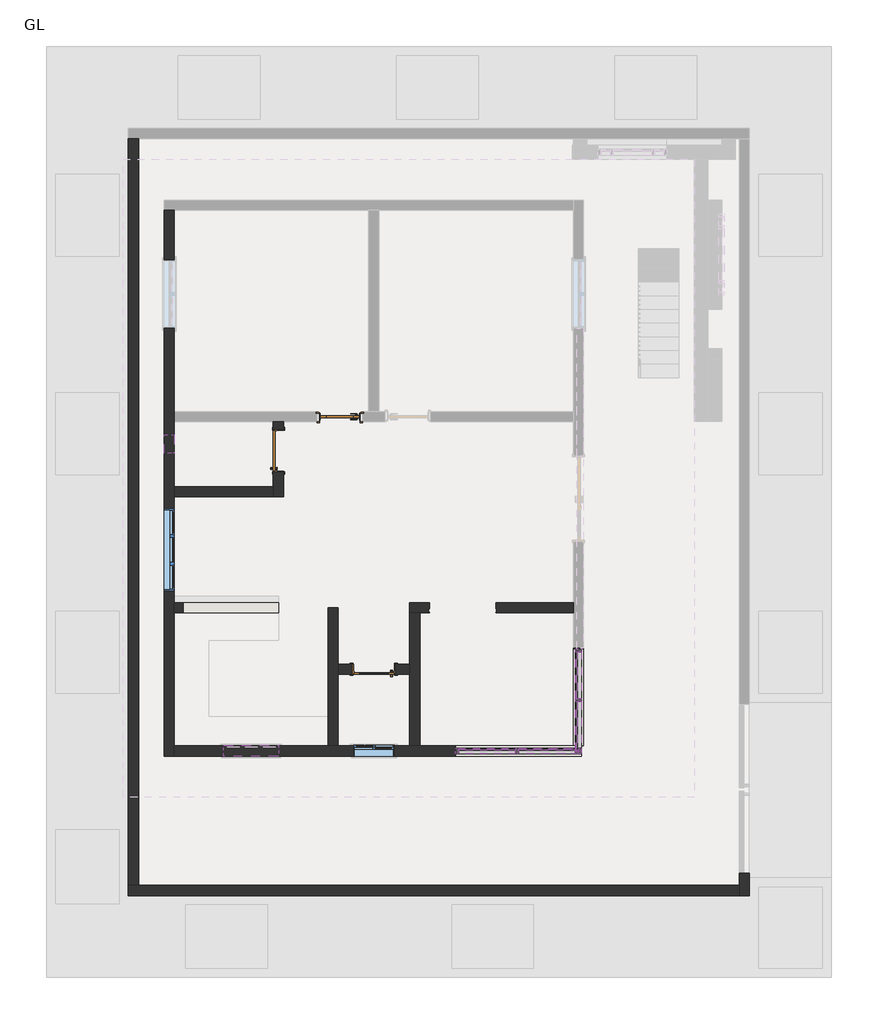
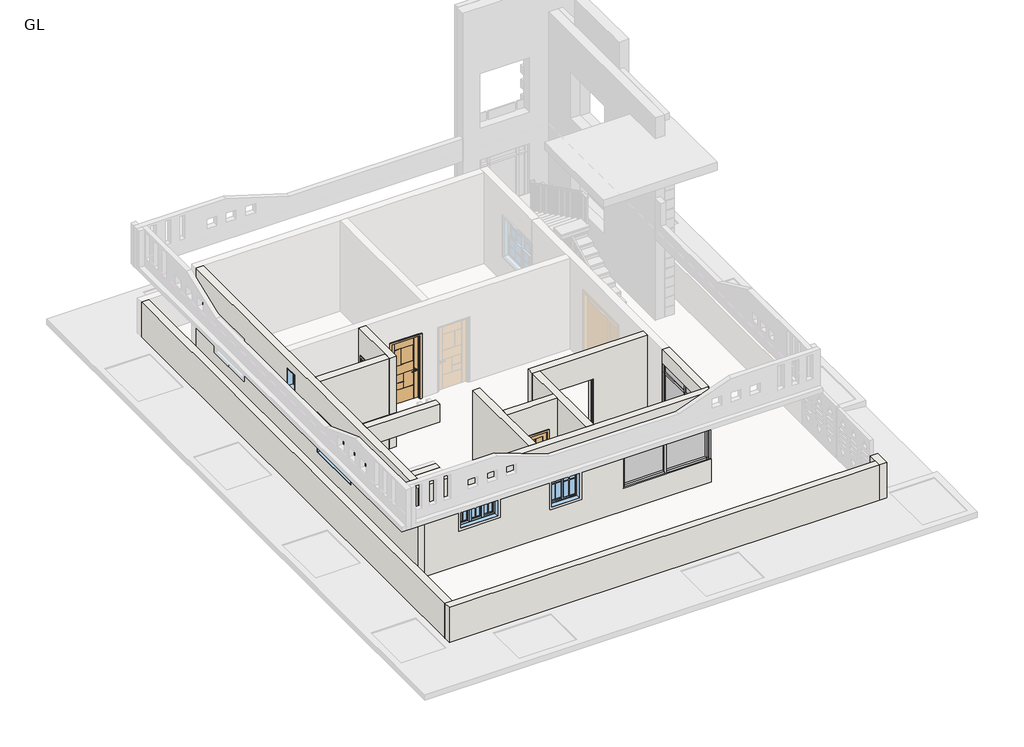
# One storey, part 1 of 4: 24 members, 13 walls, 8 plates, 4 windows, 3 doors.
"""IFC4 building model written with IfcOpenShell, lengths in millimetres."""

from ifc_helpers import new_model, si_unit, frame, origin, origin_with_axes, place, context, project, spatial, polyline, outline, extrude, faceted_brep, transform, mapped, element, save
from components import door_1d7b229f, door_d5d480c1, single_modern_wooden_door_17379_single_modern_wooden_door_9761f21e, member_cba00588, member_58fbc06e, member_82905deb, member_75d1e245, member_3c3dc66a, member_4491d118, member_78934672, member_697f972d, member_ecafcbb3, member_c327c56d, member_aaf6ec4e, member_7ce6cacc, member_69204bcc, member_41dcc1f0, system_panel_glazed_27c3d98e, system_panel_glazed_8e393102, system_panel_glazed_36abd0f2, system_panel_glazed_6ba3ac31, system_panel_glazed_448caaff, system_panel_glazed_d7074436, system_panel_glazed_2854df63, system_panel_glazed_f3e19b1d, window_aa618e30, window_06177765, window_dd70d674, window_fdfe0ef3

model = new_model("IFC4")

# Units and contexts
model_context = context("Model", 3, world=origin())
ifc_project = project(units=[si_unit("LENGTHUNIT", "METRE", prefix="MILLI")], contexts=[model_context])

# Site, building, storey
site = spatial("IfcSite", under=ifc_project)
building = spatial("IfcBuilding", under=site)
storey = spatial("IfcBuildingStorey", under=building, Name="GL", Elevation=0.0)

# Doors
placement = place(None, origin())
door_shape = door_1d7b229f(model_context)
element("IfcDoor", 1, ObjectType="Door-Interior-Single-Flush_Panel-Wood : 36\" x 84\"", at=placement, inside=storey, context=model_context, shape_type="MappedRepresentation", body=[
    mapped(door_shape, transform((-9036.4027598, 5465.7342801, 0.0), x_axis=(0.0, 1.0, 0.0), y_axis=(-1.0, 0.0, 0.0), z_axis=(0.0, 0.0, 1.0))),
])
door_2_shape = door_d5d480c1(model_context)
element("IfcDoor", 2, ObjectType="Door-Interior-Single-Full Glass-Wood : 36\" x 80\"", at=placement, inside=storey, context=model_context, shape_type="MappedRepresentation", body=[
    mapped(door_2_shape, transform((-6899.6277598, 585.7592801, 0.0), x_axis=(-1.0, 0.0, 0.0), y_axis=(0.0, -1.0, 0.0), z_axis=(0.0, 0.0, 1.0))),
])
single_modern_wooden_door_17379_single_modern_wooden_door_shape = single_modern_wooden_door_17379_single_modern_wooden_door_9761f21e(model_context)
element("IfcDoor", 3, ObjectType="Single_-_Modern_Wooden_Door_17379 : Single_-_Modern_Wooden_Door_17379", at=placement, inside=storey, context=model_context, shape_type="MappedRepresentation", body=[
    mapped(single_modern_wooden_door_17379_single_modern_wooden_door_shape, transform((-7661.6277598, 6227.7342801, 0.0), x_axis=(1.0, 0.0, 0.0), y_axis=(0.0, 1.0, 0.0), z_axis=(0.0, 0.0, 1.0))),
])

# Members
member_shape = member_cba00588(model_context)
element("IfcMember", 4, ObjectType="Rectangular Mullion : 2.5\" x 5\" rectangular", at=placement, inside=storey, context=model_context, shape_type="MappedRepresentation", body=[
    mapped(member_shape, transform((-3730.9777598, -1239.8657199, 2590.8), x_axis=(0.0, 0.0, 1.0), y_axis=(0.0, -1.0, 0.0), z_axis=(1.0, 0.0, 0.0))),
])
element("IfcMember", 5, ObjectType="Rectangular Mullion : 2.5\" x 5\" rectangular", at=placement, inside=storey, context=model_context, shape_type="MappedRepresentation", body=[
    mapped(member_shape, transform((-5007.3277598, -1239.8657199, 762.0), x_axis=(0.0, 0.0, -1.0), y_axis=(0.0, -1.0, 0.0), z_axis=(-1.0, 0.0, 0.0))),
])
member_2_shape = member_58fbc06e(model_context)
element("IfcMember", 6, ObjectType="Rectangular Mullion : 2.5\" x 5\" rectangular", at=placement, inside=storey, context=model_context, shape_type="MappedRepresentation", body=[
    mapped(member_2_shape, transform((-3730.9777598, -1239.8657199, 2286.0), x_axis=(0.0, 0.0, 1.0), y_axis=(0.0, -1.0, 0.0), z_axis=(1.0, 0.0, 0.0))),
])
member_3_shape = member_82905deb(model_context)
element("IfcMember", 7, ObjectType="Rectangular Mullion : 2.5\" x 5\" rectangular", at=placement, inside=storey, context=model_context, shape_type="MappedRepresentation", body=[
    mapped(member_3_shape, transform((-3699.2277598, -1239.8657199, 762.0), x_axis=(1.0, 0.0, 0.0), y_axis=(0.0, -1.0, 0.0), z_axis=(0.0, 0.0, -1.0))),
])
element("IfcMember", 8, ObjectType="Rectangular Mullion : 2.5\" x 5\" rectangular", at=placement, inside=storey, context=model_context, shape_type="MappedRepresentation", body=[
    mapped(member_3_shape, transform((-2327.6277598, -96.8657199, 762.0), x_axis=(0.0, 1.0, 0.0), y_axis=(1.0, 0.0, 0.0), z_axis=(0.0, 0.0, -1.0))),
])
member_4_shape = member_75d1e245(model_context)
element("IfcMember", 9, ObjectType="Rectangular Mullion : 2.5\" x 5\" rectangular", at=placement, inside=storey, context=model_context, shape_type="MappedRepresentation", body=[
    mapped(member_4_shape, transform((-3699.2277598, -1239.8657199, 2286.0), x_axis=(1.0, 0.0, 0.0), y_axis=(0.0, -1.0, 0.0), z_axis=(0.0, 0.0, -1.0))),
])
element("IfcMember", 10, ObjectType="Rectangular Mullion : 2.5\" x 5\" rectangular", at=placement, inside=storey, context=model_context, shape_type="MappedRepresentation", body=[
    mapped(member_4_shape, transform((-2327.6277598, -96.8657199, 2286.0), x_axis=(0.0, 1.0, 0.0), y_axis=(1.0, 0.0, 0.0), z_axis=(0.0, 0.0, -1.0))),
])
member_5_shape = member_3c3dc66a(model_context)
element("IfcMember", 11, ObjectType="Rectangular Mullion : 2.5\" x 5\" rectangular", at=placement, inside=storey, context=model_context, shape_type="MappedRepresentation", body=[
    mapped(member_5_shape, transform((-5070.8277598, -1239.8657199, 2590.8), x_axis=(-1.0, 0.0, 0.0), y_axis=(0.0, -1.0, 0.0), z_axis=(0.0, 0.0, 1.0))),
])
element("IfcMember", 12, ObjectType="Rectangular Mullion : 2.5\" x 5\" rectangular", at=placement, inside=storey, context=model_context, shape_type="MappedRepresentation", body=[
    mapped(member_5_shape, transform((-2327.6277598, -1303.3657199, 2590.8), x_axis=(0.0, -1.0, 0.0), y_axis=(1.0, 0.0, 0.0), z_axis=(0.0, 0.0, 1.0))),
])
member_6_shape = member_4491d118(model_context)
element("IfcMember", 13, ObjectType="Rectangular Mullion : 2.5\" x 5\" rectangular", at=placement, inside=storey, context=model_context, shape_type="MappedRepresentation", body=[
    mapped(member_6_shape, transform((-2327.6277598, 1046.1342801, 762.0), x_axis=(0.0, 1.0, 0.0), y_axis=(1.0, 0.0, 0.0), z_axis=(0.0, 0.0, -1.0))),
])
element("IfcMember", 14, ObjectType="Rectangular Mullion : 2.5\" x 5\" rectangular", at=placement, inside=storey, context=model_context, shape_type="MappedRepresentation", body=[
    mapped(member_5_shape, transform((-2327.6277598, 1046.1342801, 2286.0), x_axis=(0.0, 1.0, 0.0), y_axis=(1.0, 0.0, 0.0), z_axis=(0.0, 0.0, -1.0))),
])
element("IfcMember", 15, ObjectType="Rectangular Mullion : 2.5\" x 5\" rectangular", at=placement, inside=storey, context=model_context, shape_type="MappedRepresentation", body=[
    mapped(member_6_shape, transform((-5070.8277598, -1239.8657199, 2286.0), x_axis=(-1.0, 0.0, 0.0), y_axis=(0.0, -1.0, 0.0), z_axis=(0.0, 0.0, 1.0))),
])
element("IfcMember", 16, ObjectType="Rectangular Mullion : 2.5\" x 5\" rectangular", at=placement, inside=storey, context=model_context, shape_type="MappedRepresentation", body=[
    mapped(member_6_shape, transform((-2327.6277598, -1303.3657199, 2286.0), x_axis=(0.0, -1.0, 0.0), y_axis=(1.0, 0.0, 0.0), z_axis=(0.0, 0.0, 1.0))),
])
member_7_shape = member_78934672(model_context)
element("IfcMember", 17, ObjectType="Rectangular Mullion : 2.5\" x 5\" rectangular", at=placement, inside=storey, context=model_context, shape_type="MappedRepresentation", body=[
    mapped(member_7_shape, transform((-2327.6277598, 982.6342801, 2590.8), x_axis=(0.0, 0.0, 1.0), y_axis=(1.0, 0.0, 0.0), z_axis=(0.0, 1.0, 0.0))),
])
element("IfcMember", 18, ObjectType="Rectangular Mullion : 2.5\" x 5\" rectangular", at=placement, inside=storey, context=model_context, shape_type="MappedRepresentation", body=[
    mapped(member_7_shape, transform((-2327.6277598, -65.1157199, 762.0), x_axis=(0.0, 0.0, -1.0), y_axis=(1.0, 0.0, 0.0), z_axis=(0.0, -1.0, 0.0))),
])
member_8_shape = member_697f972d(model_context)
element("IfcMember", 19, ObjectType="Rectangular Mullion : 2.5\" x 5\" rectangular", at=placement, inside=storey, context=model_context, shape_type="MappedRepresentation", body=[
    mapped(member_8_shape, transform((-2327.6277598, 982.6342801, 2286.0), x_axis=(0.0, 0.0, 1.0), y_axis=(1.0, 0.0, 0.0), z_axis=(0.0, 1.0, 0.0))),
])
member_9_shape = member_ecafcbb3(model_context)
element("IfcMember", 20, ObjectType="Rectangular Mullion : 2.5\" x 5\" rectangular", at=placement, inside=storey, context=model_context, shape_type="MappedRepresentation", body=[
    mapped(member_9_shape, transform((-2264.1277598, -1239.8657199, 762.0), x_axis=(1.0, 0.0, 0.0), y_axis=(0.0, -1.0, 0.0), z_axis=(0.0, 0.0, -1.0))),
])
member_10_shape = member_c327c56d(model_context)
element("IfcMember", 21, ObjectType="Rectangular Mullion : 2.5\" x 5\" rectangular", at=placement, inside=storey, context=model_context, shape_type="MappedRepresentation", body=[
    mapped(member_10_shape, transform((-2264.1277598, -1239.8657199, 2317.75), x_axis=(1.0, 0.0, 0.0), y_axis=(0.0, -1.0, 0.0), z_axis=(0.0, 0.0, -1.0))),
])
member_11_shape = member_aaf6ec4e(model_context)
element("IfcMember", 22, ObjectType="Rectangular Mullion : 2.5\" x 5\" rectangular", at=placement, inside=storey, context=model_context, shape_type="MappedRepresentation", body=[
    mapped(member_11_shape, transform((-2327.6277598, -1239.8657199, 762.0), x_axis=(0.0, 0.0, -1.0), y_axis=(1.0, 0.0, 0.0), z_axis=(0.0, -1.0, 0.0))),
])
member_12_shape = member_7ce6cacc(model_context)
element("IfcMember", 23, ObjectType="Rectangular Mullion : 2.5\" x 5\" rectangular", at=placement, inside=storey, context=model_context, shape_type="MappedRepresentation", body=[
    mapped(member_12_shape, transform((-2327.6277598, -128.6157199, 2286.0), x_axis=(0.0, 0.0, 1.0), y_axis=(1.0, 0.0, 0.0), z_axis=(0.0, 1.0, 0.0))),
])
element("IfcMember", 24, ObjectType="Rectangular Mullion : 2.5\" x 5\" rectangular", at=placement, inside=storey, context=model_context, shape_type="MappedRepresentation", body=[
    mapped(member_11_shape, transform((-2327.6277598, -128.6157199, 2590.8), x_axis=(0.0, 0.0, 1.0), y_axis=(1.0, 0.0, 0.0), z_axis=(0.0, 1.0, 0.0))),
])
member_13_shape = member_69204bcc(model_context)
element("IfcMember", 25, ObjectType="Rectangular Mullion : 2.5\" x 5\" rectangular", at=placement, inside=storey, context=model_context, shape_type="MappedRepresentation", body=[
    mapped(member_13_shape, transform((-2327.6277598, -1239.8657199, 2590.8), x_axis=(0.0, 0.0, 1.0), y_axis=(0.0, -1.0, 0.0), z_axis=(1.0, 0.0, 0.0))),
])
member_14_shape = member_41dcc1f0(model_context)
element("IfcMember", 26, ObjectType="Rectangular Mullion : 2.5\" x 5\" rectangular", at=placement, inside=storey, context=model_context, shape_type="MappedRepresentation", body=[
    mapped(member_14_shape, transform((-2264.1277598, -1239.8657199, 2286.0), x_axis=(0.0, 0.0, 1.0), y_axis=(0.0, -1.0, 0.0), z_axis=(1.0, 0.0, 0.0))),
])
element("IfcMember", 27, ObjectType="Rectangular Mullion : 2.5\" x 5\" rectangular", at=placement, inside=storey, context=model_context, shape_type="MappedRepresentation", body=[
    mapped(member_13_shape, transform((-3667.4777598, -1239.8657199, 762.0), x_axis=(0.0, 0.0, -1.0), y_axis=(0.0, -1.0, 0.0), z_axis=(-1.0, 0.0, 0.0))),
])

# Plates
system_panel_glazed_shape = system_panel_glazed_27c3d98e(model_context)
element("IfcPlate", 28, ObjectType="System Panel : Glazed", at=placement, inside=storey, context=model_context, shape_type="MappedRepresentation", body=[
    mapped(system_panel_glazed_shape, transform((-4369.1527598, -1239.8657199, 825.5), x_axis=(1.0, 0.0, 0.0), y_axis=(0.0, 1.0, 0.0), z_axis=(0.0, 0.0, 1.0))),
])
system_panel_glazed_2_shape = system_panel_glazed_8e393102(model_context)
element("IfcPlate", 29, ObjectType="System Panel : Glazed", at=placement, inside=storey, context=model_context, shape_type="MappedRepresentation", body=[
    mapped(system_panel_glazed_2_shape, transform((-4369.1527598, -1239.8657199, 2317.75), x_axis=(1.0, 0.0, 0.0), y_axis=(0.0, 1.0, 0.0), z_axis=(0.0, 0.0, 1.0))),
])
system_panel_glazed_3_shape = system_panel_glazed_36abd0f2(model_context)
element("IfcPlate", 30, ObjectType="System Panel : Glazed", at=placement, inside=storey, context=model_context, shape_type="MappedRepresentation", body=[
    mapped(system_panel_glazed_3_shape, transform((-2327.6277598, 458.7592801, 825.5), x_axis=(0.0, 1.0, 0.0), y_axis=(-1.0, 0.0, 0.0), z_axis=(0.0, 0.0, 1.0))),
])
system_panel_glazed_4_shape = system_panel_glazed_6ba3ac31(model_context)
element("IfcPlate", 31, ObjectType="System Panel : Glazed", at=placement, inside=storey, context=model_context, shape_type="MappedRepresentation", body=[
    mapped(system_panel_glazed_4_shape, transform((-2327.6277598, 458.7592801, 2317.75), x_axis=(0.0, 1.0, 0.0), y_axis=(-1.0, 0.0, 0.0), z_axis=(0.0, 0.0, 1.0))),
])
system_panel_glazed_5_shape = system_panel_glazed_448caaff(model_context)
element("IfcPlate", 32, ObjectType="System Panel : Glazed", at=placement, inside=storey, context=model_context, shape_type="MappedRepresentation", body=[
    mapped(system_panel_glazed_5_shape, transform((-2327.6277598, -684.2407199, 825.5), x_axis=(0.0, 1.0, 0.0), y_axis=(-1.0, 0.0, 0.0), z_axis=(0.0, 0.0, 1.0))),
])
system_panel_glazed_6_shape = system_panel_glazed_d7074436(model_context)
element("IfcPlate", 33, ObjectType="System Panel : Glazed", at=placement, inside=storey, context=model_context, shape_type="MappedRepresentation", body=[
    mapped(system_panel_glazed_6_shape, transform((-2327.6277598, -684.2407199, 2317.75), x_axis=(0.0, 1.0, 0.0), y_axis=(-1.0, 0.0, 0.0), z_axis=(0.0, 0.0, 1.0))),
])
system_panel_glazed_7_shape = system_panel_glazed_2854df63(model_context)
element("IfcPlate", 34, ObjectType="System Panel : Glazed", at=placement, inside=storey, context=model_context, shape_type="MappedRepresentation", body=[
    mapped(system_panel_glazed_7_shape, transform((-2997.5527598, -1239.8657199, 825.5), x_axis=(1.0, 0.0, 0.0), y_axis=(0.0, 1.0, 0.0), z_axis=(0.0, 0.0, 1.0))),
])
system_panel_glazed_8_shape = system_panel_glazed_f3e19b1d(model_context)
element("IfcPlate", 35, ObjectType="System Panel : Glazed", at=placement, inside=storey, context=model_context, shape_type="MappedRepresentation", body=[
    mapped(system_panel_glazed_8_shape, transform((-2997.5527598, -1239.8657199, 2317.75), x_axis=(1.0, 0.0, 0.0), y_axis=(0.0, 1.0, 0.0), z_axis=(0.0, 0.0, 1.0))),
])

# Walls
element("IfcWall", 36, ObjectType="Generic - 9\"", at=placement, inside=storey, context=model_context, shape_type="Brep", body=[
    faceted_brep([(-11357.3277598, -1354.1657199, 0.0), (-11357.3277598, -1125.5657199, 0.0), (-11357.3277598, 1846.2342801, 0.0), (-11357.3277598, 2074.8342801, 0.0), (-11357.3277598, 4437.0342801, 0.0), (-11357.3277598, 4665.6342801, 0.0), (-11357.3277598, 6113.4342801, 0.0), (-11357.3277598, 6342.0342801, 0.0), (-11357.3277598, 10837.8342801, 0.0), (-11357.3277598, 10837.8342801, 3048.0), (-11357.3277598, 6342.0342801, 3048.0), (-11357.3277598, 6113.4342801, 3048.0), (-11357.3277598, 4665.6342801, 3048.0), (-11357.3277598, 4437.0342801, 3048.0), (-11357.3277598, 2074.8342801, 3048.0), (-11357.3277598, 1846.2342801, 3048.0), (-11357.3277598, -1125.5657199, 3048.0), (-11357.3277598, -1354.1657199, 3048.0), (-11357.3277598, 9732.9342801, 2235.2), (-11357.3277598, 9732.9342801, 914.4), (-11357.3277598, 8208.9342801, 914.4), (-11357.3277598, 8208.9342801, 2235.2), (-11357.3277598, 2341.5342801, 2260.6), (-11357.3277598, 4170.3342801, 2260.6), (-11357.3277598, 4170.3342801, 914.4), (-11357.3277598, 2341.5342801, 914.4), (-11357.3277598, 5414.9342801, 2743.2), (-11357.3277598, 5821.3342801, 2743.2), (-11357.3277598, 5821.3342801, 2133.6), (-11357.3277598, 5414.9342801, 2133.6), (-11585.9277598, -1354.1657199, 0.0), (-11585.9277598, -1354.1657199, 3048.0), (-11585.9277598, 10837.8342801, 3048.0), (-11585.9277598, 10837.8342801, 0.0), (-11585.9277598, 9732.9342801, 2235.2), (-11585.9277598, 8208.9342801, 2235.2), (-11585.9277598, 8208.9342801, 914.4), (-11585.9277598, 9732.9342801, 914.4), (-11585.9277598, 2341.5342801, 2260.6), (-11585.9277598, 2341.5342801, 914.4), (-11585.9277598, 4170.3342801, 914.4), (-11585.9277598, 4170.3342801, 2260.6), (-11585.9277598, 5414.9342801, 2743.2), (-11585.9277598, 5414.9342801, 2133.6), (-11585.9277598, 5821.3342801, 2133.6), (-11585.9277598, 5821.3342801, 2743.2)], [[[0, 1, 2, 3, 4, 5, 6, 7, 8, 9, 10, 11, 12, 13, 14, 15, 16, 17], [18, 19, 20, 21], [22, 23, 24, 25], [26, 27, 28, 29]], [[30, 31, 32, 33], [34, 35, 36, 37], [38, 39, 40, 41], [42, 43, 44, 45]], [[8, 7, 6, 5, 4, 3, 2, 1, 0, 30, 33]], [[17, 16, 15, 14, 13, 12, 11, 10, 9, 32, 31]], [[0, 17, 31, 30]], [[9, 8, 33, 32]], [[19, 18, 34, 37]], [[20, 19, 37, 36]], [[21, 20, 36, 35]], [[18, 21, 35, 34]], [[39, 38, 22, 25]], [[40, 39, 25, 24]], [[41, 40, 24, 23]], [[38, 41, 23, 22]], [[43, 42, 26, 29]], [[44, 43, 29, 28]], [[45, 44, 28, 27]], [[42, 45, 27, 26]]]),
])
element("IfcWall", 37, ObjectType="Generic - 9\"", at=placement, inside=storey, context=model_context, shape_type="Brep", body=[
    faceted_brep([(-2264.1277598, -1125.5657199, 2590.8), (-2441.9277598, -1125.5657199, 2590.8), (-5070.8277598, -1125.5657199, 2590.8), (-5070.8277598, -1125.5657199, 762.0), (-2441.9277598, -1125.5657199, 762.0), (-2264.1277598, -1125.5657199, 762.0), (-2264.1277598, -1125.5657199, 0.0), (-2441.9277598, -1125.5657199, 0.0), (-5870.9277598, -1125.5657199, 0.0), (-6099.5277598, -1125.5657199, 0.0), (-7699.7277598, -1125.5657199, 0.0), (-7928.3277598, -1125.5657199, 0.0), (-11357.3277598, -1125.5657199, 0.0), (-11357.3277598, -1125.5657199, 3048.0), (-7928.3277598, -1125.5657199, 3048.0), (-7699.7277598, -1125.5657199, 3048.0), (-6099.5277598, -1125.5657199, 3048.0), (-5870.9277598, -1125.5657199, 3048.0), (-2441.9277598, -1125.5657199, 3048.0), (-2264.1277598, -1125.5657199, 3048.0), (-9033.2277598, -1125.5657199, 2133.6), (-10252.4277598, -1125.5657199, 2133.6), (-10252.4277598, -1125.5657199, 1219.2), (-9033.2277598, -1125.5657199, 1219.2), (-6442.4277598, -1125.5657199, 2133.6), (-7356.8277598, -1125.5657199, 2133.6), (-7356.8277598, -1125.5657199, 914.4), (-6442.4277598, -1125.5657199, 914.4), (-2264.1277598, -1354.1657199, 2590.8), (-2264.1277598, -1354.1657199, 3048.0), (-11357.3277598, -1354.1657199, 3048.0), (-11357.3277598, -1354.1657199, 0.0), (-2264.1277598, -1354.1657199, 0.0), (-2264.1277598, -1354.1657199, 762.0), (-5070.8277598, -1354.1657199, 762.0), (-5070.8277598, -1354.1657199, 2590.8), (-9033.2277598, -1354.1657199, 2133.6), (-9033.2277598, -1354.1657199, 1219.2), (-10252.4277598, -1354.1657199, 1219.2), (-10252.4277598, -1354.1657199, 2133.6), (-6442.4277598, -1354.1657199, 2133.6), (-6442.4277598, -1354.1657199, 914.4), (-7356.8277598, -1354.1657199, 914.4), (-7356.8277598, -1354.1657199, 2133.6)], [[[0, 1, 2, 3, 4, 5, 6, 7, 8, 9, 10, 11, 12, 13, 14, 15, 16, 17, 18, 19], [20, 21, 22, 23], [24, 25, 26, 27]], [[28, 29, 30, 31, 32, 33, 34, 35], [36, 37, 38, 39], [40, 41, 42, 43]], [[13, 12, 31, 30]], [[37, 36, 20, 23]], [[38, 37, 23, 22]], [[39, 38, 22, 21]], [[36, 39, 21, 20]], [[41, 40, 24, 27]], [[42, 41, 27, 26]], [[43, 42, 26, 25]], [[40, 43, 25, 24]], [[12, 11, 10, 9, 8, 7, 6, 32, 31]], [[19, 18, 17, 16, 15, 14, 13, 30, 29]], [[0, 19, 29, 28]], [[2, 1, 0, 28, 35]], [[3, 2, 35, 34]], [[5, 4, 3, 34, 33]], [[6, 5, 33, 32]]]),
])
element("IfcWall", 38, ObjectType="Generic - 9\"", at=placement, inside=storey, context=model_context, shape_type="SweptSolid", body=[
    extrude(outline(polyline([(0.0, -11357.3277598), (0.0, -9033.2277598), (914.4, -9033.2277598), (914.4, -11166.8277598), (2438.4, -11166.8277598), (2438.4, -9033.2277598), (3048.0, -9033.2277598), (3048.0, -11357.3277598), (0.0, -11357.3277598)])), frame((0.0, 1846.2342801, 0.0), z_axis=(0.0, 1.0, 0.0), x_axis=(0.0, 0.0, 1.0)), (0.0, 0.0, 1.0), 228.6),
])
element("IfcWall", 39, ObjectType="Generic - 9\"", at=placement, inside=storey, context=model_context, shape_type="Brep", body=[
    faceted_brep([(-7928.3277598, 1960.5342801, 0.0), (-7928.3277598, -1125.5657199, 0.0), (-7928.3277598, -1125.5657199, 3048.0), (-7928.3277598, 1960.5342801, 3048.0), (-7699.7277598, 1960.5342801, 0.0), (-7699.7277598, 1960.5342801, 3048.0), (-7699.7277598, 703.2342801, 3048.0), (-7699.7277598, 474.6342801, 3048.0), (-7699.7277598, -1125.5657199, 3048.0), (-7699.7277598, -1125.5657199, 0.0), (-7699.7277598, 474.6342801, 0.0), (-7699.7277598, 703.2342801, 0.0)], [[[0, 1, 2, 3]], [[4, 5, 6, 7, 8, 9, 10, 11]], [[1, 0, 4, 11, 10, 9]], [[3, 2, 8, 7, 6, 5]], [[0, 3, 5, 4]], [[2, 1, 9, 8]]]),
])
element("IfcWall", 40, ObjectType="Generic - 9\"", at=placement, inside=storey, context=model_context, shape_type="SweptSolid", body=[
    extrude(outline(polyline([(3048.0, -6099.5277598), (3048.0, -7699.7277598), (0.0, -7699.7277598), (0.0, -7382.2277598), (2057.4, -7382.2277598), (2057.4, -6417.0277598), (0.0, -6417.0277598), (0.0, -6099.5277598), (3048.0, -6099.5277598)])), frame((0.0, 474.6342801, 0.0), z_axis=(0.0, 1.0, 0.0), x_axis=(0.0, 0.0, 1.0)), (0.0, 0.0, 1.0), 228.6),
])
element("IfcWall", 41, ObjectType="Generic - 9\"", at=placement, inside=storey, context=model_context, shape_type="Brep", body=[
    faceted_brep([(-6099.5277598, 1846.2342801, 0.0), (-6099.5277598, 703.2342801, 0.0), (-6099.5277598, 474.6342801, 0.0), (-6099.5277598, -1125.5657199, 0.0), (-6099.5277598, -1125.5657199, 3048.0), (-6099.5277598, 474.6342801, 3048.0), (-6099.5277598, 703.2342801, 3048.0), (-6099.5277598, 1846.2342801, 3048.0), (-5870.9277598, 1846.2342801, 0.0), (-5870.9277598, 1846.2342801, 3048.0), (-5870.9277598, -1125.5657199, 3048.0), (-5870.9277598, -1125.5657199, 0.0)], [[[0, 1, 2, 3, 4, 5, 6, 7]], [[8, 9, 10, 11]], [[3, 2, 1, 0, 8, 11]], [[7, 6, 5, 4, 10, 9]], [[4, 3, 11, 10]], [[0, 7, 9, 8]]]),
])
element("IfcWall", 42, ObjectType="Generic - 9\"", at=placement, inside=storey, context=model_context, shape_type="Brep", body=[
    faceted_brep([(-6099.5277598, 2074.8342801, 3048.0), (-2441.9277598, 2074.8342801, 3048.0), (-2441.9277598, 2074.8342801, 0.0), (-4175.9277598, 2074.8342801, 0.0), (-4175.9277598, 2074.8342801, 2189.5), (-5660.9277598, 2074.8342801, 2189.5), (-5660.9277598, 2074.8342801, 0.0), (-6099.5277598, 2074.8342801, 0.0), (-2441.9277598, 1846.2342801, 3048.0), (-5870.9277598, 1846.2342801, 3048.0), (-6099.5277598, 1846.2342801, 3048.0), (-6099.5277598, 1846.2342801, 0.0), (-5870.9277598, 1846.2342801, 0.0), (-5660.9277598, 1846.2342801, 0.0), (-5660.9277598, 1846.2342801, 2189.5), (-4175.9277598, 1846.2342801, 2189.5), (-4175.9277598, 1846.2342801, 0.0), (-2441.9277598, 1846.2342801, 0.0), (-4175.9277598, 1866.2342801, 0.0), (-4160.9277598, 1866.2342801, 0.0), (-4160.9277598, 1943.2342801, 0.0), (-4175.9277598, 1943.2342801, 0.0), (-5660.9277598, 1943.2342801, 0.0), (-5675.9277598, 1943.2342801, 0.0), (-5675.9277598, 1866.2342801, 0.0), (-5660.9277598, 1866.2342801, 0.0), (-4175.9277598, 1866.2342801, 2189.5), (-5660.9277598, 1866.2342801, 2189.5), (-5675.9277598, 1866.2342801, 2204.5), (-4160.9277598, 1866.2342801, 2204.5), (-4160.9277598, 1943.2342801, 2204.5), (-5675.9277598, 1943.2342801, 2204.5), (-5660.9277598, 1943.2342801, 2189.5), (-4175.9277598, 1943.2342801, 2189.5)], [[[0, 1, 2, 3, 4, 5, 6, 7]], [[8, 9, 10, 11, 12, 13, 14, 15, 16, 17]], [[2, 17, 16, 18, 19, 20, 21, 3]], [[11, 7, 6, 22, 23, 24, 25, 13, 12]], [[1, 0, 10, 9, 8]], [[2, 1, 8, 17]], [[0, 7, 11, 10]], [[26, 18, 16, 15]], [[25, 27, 14, 13]], [[27, 26, 15, 14]], [[18, 26, 27, 25, 24, 28, 29, 19]], [[19, 29, 30, 20]], [[20, 30, 31, 23, 22, 32, 33, 21]], [[29, 28, 31, 30]], [[28, 24, 23, 31]], [[21, 33, 4, 3]], [[32, 22, 6, 5]], [[33, 32, 5, 4]]]),
])
element("IfcWall", 43, ObjectType="Generic - 9\"", at=placement, inside=storey, context=model_context, shape_type="Brep", body=[
    faceted_brep([(-9147.5277598, 4437.0342801, 3048.0), (-9147.5277598, 4665.6342801, 3048.0), (-9147.5277598, 6113.4342801, 3048.0), (-9147.5277598, 6113.4342801, 0.0), (-9147.5277598, 5948.3342801, 0.0), (-9147.5277598, 5948.3342801, 2159.0), (-9147.5277598, 4983.1342801, 2159.0), (-9147.5277598, 4983.1342801, 0.0), (-9147.5277598, 4665.6342801, 0.0), (-9147.5277598, 4437.0342801, 0.0), (-8918.9277598, 6113.4342801, 3048.0), (-8918.9277598, 4437.0342801, 3048.0), (-8918.9277598, 4437.0342801, 0.0), (-8918.9277598, 4983.1342801, 0.0), (-8918.9277598, 4983.1342801, 2159.0), (-8918.9277598, 5948.3342801, 2159.0), (-8918.9277598, 5948.3342801, 0.0), (-8918.9277598, 6113.4342801, 0.0)], [[[0, 1, 2, 3, 4, 5, 6, 7, 8, 9]], [[10, 11, 12, 13, 14, 15, 16, 17]], [[3, 17, 16, 4]], [[12, 9, 8, 7, 13]], [[2, 1, 0, 11, 10]], [[3, 2, 10, 17]], [[0, 9, 12, 11]], [[15, 5, 4, 16]], [[5, 15, 14, 6]], [[6, 14, 13, 7]]]),
])
element("IfcWall", 44, ObjectType="Generic - 9\"", at=placement, inside=storey, context=model_context, shape_type="SweptSolid", body=[
    extrude(outline(polyline([(-11357.3277598, 4665.6342801), (-9147.5277598, 4665.6342801), (-9147.5277598, 4437.0342801), (-11357.3277598, 4437.0342801), (-11357.3277598, 4665.6342801)])), origin_with_axes(), (0.0, 0.0, 1.0), 3048.0),
])
element("IfcWall", 45, ObjectType="Generic - 9\"", at=placement, inside=storey, context=model_context, shape_type="Brep", body=[
    faceted_brep([(1266.4722402, -4237.0657199, 0.0), (-12157.4277598, -4237.0657199, 0.0), (-12386.0277598, -4237.0657199, 0.0), (-12386.0277598, -4237.0657199, 1219.2), (-12157.4277598, -4237.0657199, 1219.2), (1266.4722402, -4237.0657199, 1219.2), (1266.4722402, -4465.6657199, 0.0), (1266.4722402, -4465.6657199, 1219.2), (-12386.0277598, -4465.6657199, 1219.2), (-12386.0277598, -4465.6657199, 0.0)], [[[0, 1, 2, 3, 4, 5]], [[6, 7, 8, 9]], [[2, 1, 0, 6, 9]], [[5, 4, 3, 8, 7]], [[0, 5, 7, 6]], [[3, 2, 9, 8]]]),
])
element("IfcWall", 46, ObjectType="Generic - 9\"", at=placement, inside=storey, context=model_context, shape_type="SweptSolid", body=[
    extrude(outline(polyline([(-12157.4277598, 12438.0342801), (-12157.4277598, -4237.0657199), (-12386.0277598, -4237.0657199), (-12386.0277598, 12438.0342801), (-12157.4277598, 12438.0342801)])), origin_with_axes(), (0.0, 0.0, 1.0), 1219.2),
])
element("IfcWall", 47, ObjectType="Generic - 9\"", at=placement, inside=storey, context=model_context, shape_type="Brep", body=[
    faceted_brep([(1266.4722402, -3970.3657199, 0.0), (1266.4722402, -4237.0657199, 0.0), (1266.4722402, -4465.6657199, 0.0), (1266.4722402, -4465.6657199, 1219.2), (1266.4722402, -4237.0657199, 1219.2), (1266.4722402, -3970.3657199, 1219.2), (1495.0722402, -3970.3657199, 0.0), (1495.0722402, -3970.3657199, 1219.2), (1495.0722402, -4465.6657199, 1219.2), (1495.0722402, -4465.6657199, 0.0)], [[[0, 1, 2, 3, 4, 5]], [[6, 7, 8, 9]], [[2, 1, 0, 6, 9]], [[5, 4, 3, 8, 7]], [[0, 5, 7, 6]], [[3, 2, 9, 8]]]),
])
element("IfcWall", 48, ObjectType="Generic - 9\"", at=placement, inside=storey, context=model_context, shape_type="Brep", body=[
    faceted_brep([(-2441.9277598, -1125.5657199, 762.0), (-2441.9277598, 1046.1342801, 762.0), (-2441.9277598, 1046.1342801, 2590.8), (-2441.9277598, -1125.5657199, 2590.8), (-2441.9277598, -1125.5657199, 3048.0), (-2441.9277598, 1052.4842801, 3048.0), (-2441.9277598, 1052.4842801, 0.0), (-2441.9277598, -1125.5657199, 0.0), (-2213.3277598, -1125.5657199, 762.0), (-2213.3277598, -1125.5657199, 0.0), (-2213.3277598, 1052.4842801, 0.0), (-2213.3277598, 1052.4842801, 152.4), (-2213.3277598, 1052.4842801, 304.8), (-2213.3277598, 1052.4842801, 448.7333333), (-2213.3277598, 1052.4842801, 601.1333333), (-2213.3277598, 1052.4842801, 745.0666667), (-2213.3277598, 1052.4842801, 897.4666667), (-2213.3277598, 1052.4842801, 1041.4), (-2213.3277598, 1052.4842801, 1193.8), (-2213.3277598, 1052.4842801, 1337.7333333), (-2213.3277598, 1052.4842801, 1490.1333333), (-2213.3277598, 1052.4842801, 1634.0666667), (-2213.3277598, 1052.4842801, 1786.4666667), (-2213.3277598, 1052.4842801, 1930.4), (-2213.3277598, 1052.4842801, 2082.8), (-2213.3277598, 1052.4842801, 2226.7333333), (-2213.3277598, 1052.4842801, 2379.1333333), (-2213.3277598, 1052.4842801, 2523.0666667), (-2213.3277598, 1052.4842801, 2675.4666667), (-2213.3277598, 1052.4842801, 2819.4), (-2213.3277598, 1052.4842801, 2971.8), (-2213.3277598, 1052.4842801, 3048.0), (-2213.3277598, -1125.5657199, 3048.0), (-2213.3277598, -1125.5657199, 2590.8), (-2213.3277598, 1046.1342801, 2590.8), (-2213.3277598, 1046.1342801, 762.0), (-2264.1277598, -1125.5657199, 3048.0), (-2264.1277598, -1125.5657199, 2590.8), (-2264.1277598, -1125.5657199, 0.0), (-2264.1277598, -1125.5657199, 762.0)], [[[0, 1, 2, 3, 4, 5, 6, 7]], [[8, 9, 10, 11, 12, 13, 14, 15, 16, 17, 18, 19, 20, 21, 22, 23, 24, 25, 26, 27, 28, 29, 30, 31, 32, 33, 34, 35]], [[5, 4, 36, 32, 31]], [[3, 2, 34, 33, 37]], [[2, 1, 35, 34]], [[7, 6, 10, 9, 38]], [[1, 0, 39, 8, 35]], [[6, 5, 31, 30, 29, 28, 27, 26, 25, 24, 23, 22, 21, 20, 19, 18, 17, 16, 15, 14, 13, 12, 11, 10]], [[0, 7, 38, 9, 8, 39]], [[4, 3, 37, 33, 32, 36]]]),
])

# Windows
window_shape = window_aa618e30(model_context)
element("IfcWindow", 49, ObjectType="Fixed : 16\" x 24\"", at=placement, inside=storey, context=model_context, shape_type="MappedRepresentation", body=[
    mapped(window_shape, transform((-11471.6277598, 5580.0342801, 1219.2), x_axis=(0.0, -1.0, 0.0), y_axis=(1.0, 0.0, 0.0), z_axis=(0.0, 0.0, 1.0))),
])
window_2_shape = window_06177765(model_context)
element("IfcWindow", 50, ObjectType="Window-Awning-Triple-Horizontal : 48\" x 36\"", at=placement, inside=storey, context=model_context, shape_type="MappedRepresentation", body=[
    mapped(window_2_shape, transform((-9642.8277598, -1239.8657199, 304.8), x_axis=(1.0, 0.0, 0.0), y_axis=(0.0, 1.0, 0.0), z_axis=(0.0, 0.0, 1.0))),
])
window_3_shape = window_dd70d674(model_context)
element("IfcWindow", 51, ObjectType="Window-Casement-Triple-Side-Transom : 72\" x 53\"", at=placement, inside=storey, context=model_context, shape_type="MappedRepresentation", body=[
    mapped(window_3_shape, transform((-11471.6277598, 3255.9342801, 0.0), x_axis=(0.0, -1.0, 0.0), y_axis=(1.0, 0.0, 0.0), z_axis=(0.0, 0.0, 1.0))),
])
window_4_shape = window_fdfe0ef3(model_context)
element("IfcWindow", 52, ObjectType="Window-Sliding-Double : 36\" x 48\"", at=placement, inside=storey, context=model_context, shape_type="MappedRepresentation", body=[
    mapped(window_4_shape, transform((-6899.6277598, -1236.0557199, 0.0), x_axis=(1.0, 0.0, 0.0), y_axis=(0.0, 1.0, 0.0), z_axis=(0.0, 0.0, 1.0))),
])

save(model, "model.ifc")

# Revit data of these elements
# Type "Door-Interior-Single-Flush_Panel-Wood : 36\" x 84\""
#   Type Mark = "12"
#   Analytic Construction = "Wooden"
#   Thickness = 0' - 1 3/8"
#   Thermal Resistance (R) = 2.5876 (h·ft²·°F)/BTU
#   Swing Angle [instance default] = 90.00°
#   Rough Width = 3' - 2"
#   Rough Height = 7' - 1"
#   Height = 7' - 0"
#   Width = 3' - 0"
#   Heat Transfer Coefficient (U) = 0.3865 BTU/(h·ft²·°F)
#   Trim Material = Cherry
#   Panel Material = Cherry
#   Frame Material = Cherry
#   Door Handle Material = Aluminum
#   Visual Light Transmittance = 0
#   Solar Heat Gain Coefficient = 0
#   Wall Closure = (empty or 0)
#   Function = (empty or 0)
# Type "Door-Interior-Single-Full Glass-Wood : 36\" x 80\""
#   Type Mark = "11"
#   Analytic Construction = "Wood frame with single clear glass"
#   Top Rail = 0' - 4 11/16"
#   Thickness = 0' - 1 3/8"
#   Thermal Resistance (R) = 1.0102 (h·ft²·°F)/BTU
#   Swing Angle [instance default] = 90.00°
#   Stiles = 0' - 4 3/4"
#   Rough Width = 3' - 2"
#   Rough Height = 6' - 9"
#   Height = 6' - 8"
#   Width = 3' - 0"
#   Heat Transfer Coefficient (U) = 0.9900 BTU/(h·ft²·°F)
#   Bottom Rail = 0' - 9 1/8"
#   Show Grill [instance default] = yes
#   Trim Material = Cherry
#   Panel Material = Cherry
#   Frame Material = Cherry
#   Door Handle Material = Aluminum
#   Visual Light Transmittance = 0
#   Solar Heat Gain Coefficient = 0
#   Wall Closure = (empty or 0)
#   Function = (empty or 0)
# Type "Single_-_Modern_Wooden_Door_17379 : Single_-_Modern_Wooden_Door_17379"
#   Type Mark = "8"
#   Frame Projection Ext. = 0' - 1"
#   Frame Projection Int. = 0' - 1"
#   Frame Width = 0' - 2"
#   Height = 7' - 0"
#   Width = 3' - 0"
#   Handel = Stainless Steel AISI 304
#   Glass = Glass
#   Door Frame = Wood (Oak)
#   Door = Custom Walnut
#   Function = (empty or 0)
#   Wall Closure = (empty or 0)
# Type "Rectangular Mullion : 2.5\" x 5\" rectangular"
#   built-in parameter 1007304 = 0.416667 (stored number, unit not read)
#   built-in parameter 1007301 = 0.104167 (stored number, unit not read)
#   built-in parameter 1007300 = 0.104167 (stored number, unit not read)
# Type "System Panel : Glazed"
#   Construction Type Id = "GSP4R"
#   Analytic Construction = "1/8 in Pilkington single glazing"
#   Visual Light Transmittance = 0.9
#   Solar Heat Gain Coefficient = 0.86
#   Heat Transfer Coefficient (U) = 1.18115 BTU/(h·ft²·°F)
#   Define Thermal Properties by = 1
# Type "Generic - 9\""
#   Layers, outside or top first: 0' - 0 1/2" no material (function 4); 0' - 8" "Brick, Common" (function 1); 0' - 0 1/2" no material (function 5)
# Type "Fixed : 16\" x 24\""
#   Type Mark = "4"
#   Construction Type Id = "GSP4R"
#   Analytic Construction = "1/8 in Pilkington single glazing"
#   Visual Light Transmittance = 0.9
#   Solar Heat Gain Coefficient = 0.78
#   Heat Transfer Coefficient (U) = 0.6496 BTU/(h·ft²·°F)
#   Height = 2' - 0"
#   Default Sill Height = 3' - 0"
#   Width = 1' - 4"
#   Window Inset = 0' - 0 3/4"
#   Define Thermal Properties by = 1
#   Define Thermal Properties by = 1
#   Glass Pane Material = Glass
#   Sash Material = Sash
#   Wall Closure = (empty or 0)
# Type "Window-Awning-Triple-Horizontal : 48\" x 36\""
#   Type Mark = "24"
#   Fire Rating = "0.5h"
#   Analytic Construction = "Double glazing - domestic"
#   Window Inset [instance default] = 0' - 0"
#   Wall Thickness [instance default] = 0' - 6"
#   Muntin Width = 0' - 10.66667"
#   Visual Light Transmittance = 0.81
#   Thermal Resistance (R) = 1.8146 (h·ft²·°F)/BTU
#   Solar Heat Gain Coefficient = 0.76
#   One Third Width = 1' - 4"
#   Sash Width = 1' - 3.16667"
#   Rough Width = 4' - 0 1/2"
#   Rough Height = 3' - 0 1/2"
#   Interior Wall Closure [instance default] = 0' - 2 1/4"
#   Height = 3' - 0"
#   Heat Transfer Coefficient (U) = 0.5511 BTU/(h·ft²·°F)
#   Muntin Height = 2' - 6 1/2"
#   Frame Extension [instance default] = 0' - 0 1/4"
#   Exterior Wall Closure [instance default] = 0' - 1 1/4"
#   Extension Jamb [instance default] = 0' - 2 1/4"
#   Default Sill Height = 3' - 0"
#   Width = 4' - 0"
#   Middle Muntin Visibility = yes
#   Side Muntin Visibility = yes
#   Interior Trim Visibility [instance default] = yes
#   Exterior Trim Visibility [instance default] = yes
#   Extension Jamb Visibility [instance default] = yes
#   Muntin Pattern = Muntin Pattern_2x2 : Muntin Pattern_2x2
#   Interior Trim Material = Wood - Stained
#   Interior Trim = Trim-Window-Interior-Flat : Picture Frame
#   Interior Frame Material = Wood - Stained
#   Glass Panel Material = Glass
#   Exterior Trim Material = Clad - White
#   Exterior Trim = Trim-Window-Exterior-Flat : with Sill
#   Exterior Frame Material = Clad - White
#   Wall Closure = (empty or 0)
# Type "Window-Casement-Triple-Side-Transom : 72\" x 53\""
#   Type Mark = "19"
#   Fire Rating = "0.5h"
#   Analytic Construction = "Double glazing - domestic"
#   Window Width = 2' - 0"
#   Window Inset [instance default] = 0' - 0 5/8"
#   Wall Thickness [instance default] = 0' - 6"
#   Visual Light Transmittance = 0.81
#   Transom Height Ratio = 0.3
#   Thermal Resistance (R) = 1.8146 (h·ft²·°F)/BTU
#   Solar Heat Gain Coefficient = 0.76
#   Rough Width = 6' - 0 1/2"
#   Rough Height = 4' - 5 1/2"
#   Open Window Height = 3' - 1.1"
#   Heat Transfer Coefficient (U) = 0.5511 BTU/(h·ft²·°F)
#   Height = 4' - 5"
#   Transom Height = 1' - 3.9"
#   Frame Gap 3 [instance default] = 0' - 1 83/128"
#   Frame Gap 2 [instance default] = 0' - 0 5/8"
#   Frame Gap 1 = 0' - 1 51/128"
#   Default Sill Height = 3' - 0"
#   Width = 6' - 0"
#   Frame Material = Metal - Aluminum
#   Glass Panel Material = Glass
#   Wall Closure = (empty or 0)
# Type "Window-Sliding-Double : 36\" x 48\""
#   Type Mark = "23"
#   Fire Rating = "0.5h"
#   Analytic Construction = "Double glazing - domestic"
#   Window Inset [instance default] = 0' - 0"
#   Wall Thickness [instance default] = 0' - 6"
#   Visual Light Transmittance = 0.81
#   Thermal Resistance (R) = 1.8146 (h·ft²·°F)/BTU
#   Solar Heat Gain Coefficient = 0.76
#   Muntin Width = 1' - 2 5/8"
#   Muntin Height = 3' - 6 1/4"
#   Interior Wall Closure [instance default] = 0' - 2 3/4"
#   Heat Transfer Coefficient (U) = 0.5511 BTU/(h·ft²·°F)
#   Frame Extension [instance default] = 0' - 0 1/4"
#   Exterior Wall Closure [instance default] = 0' - 1 1/4"
#   Rough Width = 3' - 0 1/2"
#   Rough Height = 4' - 0 1/2"
#   Height = 4' - 0"
#   Extension Jamb [instance default] = 0' - 2 3/4"
#   Default Sill Height = 3' - 0"
#   Width = 3' - 0"
#   Interior Trim Visibility [instance default] = yes
#   Indicator Visibility [instance default] = yes
#   Exterior Trim Visibility [instance default] = yes
#   Muntin Visibility = yes
#   Extension Jamb Visibility [instance default] = yes
#   Muntin Pattern = Muntin Pattern_2x2 : Muntin Pattern_2x2
#   Interior Trim Material = Wood - Stained
#   Interior Trim = Trim-Window-Interior-Flat : Picture Frame
#   Interior Frame Material = Wood - Stained
#   Glass Panel Material = Glass
#   Exterior Trim Material = Clad - White
#   Exterior Trim = Trim-Window-Exterior-Flat : with Sill
#   Exterior Frame Material = Clad - White
#   Wall Closure = (empty or 0)
# Element 1 (IfcDoor, "Door-Interior-Single-Flush_Panel-Wood : 36\" x 84\"")
#   Swing Angle = 90.00°
#   Phase Created = New Construction
#   Materials on its faces: "Cherry", "Aluminum"
# Element 2 (IfcDoor, "Door-Interior-Single-Full Glass-Wood : 36\" x 80\"")
#   Swing Angle = 90.00°
#   Show Grill = yes
#   Phase Created = New Construction
#   Materials on its faces: "Cherry", "Aluminum", "Glass"
# Element 3 (IfcDoor, "Single_-_Modern_Wooden_Door_17379 : Single_-_Modern_Wooden_Door_17379")
#   Phase Created = New Construction
#   Materials on its faces: "Stainless Steel AISI 304", "Custom Walnut", "Wood (Oak)", "Glass"
# Elements 4, 5, 6, 7, 8, 9, 10, 11, 12, 13, 14, 15, 16, 17, 18, 19, 20, 21, 22, 23, 24, 25, 26, 27 (IfcMember, "Rectangular Mullion : 2.5\" x 5\" rectangular")
#   Phase Created = New Construction
#   Materials on its faces: "Aluminum"
# Elements 28, 29, 30, 31, 32, 33, 34, 35 (IfcPlate, "System Panel : Glazed")
#   Phase Created = New Construction
#   Materials on its faces: "Glass"
# Elements 36, 37, 38, 39, 40, 41, 42, 43, 44, 48 (IfcWall, "Generic - 9\"")
#   Top Offset = -0' - 6"
#   Base Offset = 0' - 0"
#   wall height = 10' - 0"
#   Phase Created = New Construction
#   Base Constraint = GL
#   Top Constraint = 1st floor
#   Materials on its faces: "Default Wall"
# Elements 45, 46, 47 (IfcWall, "Generic - 9\"")
#   Top Offset = -0' - 6"
#   Base Offset = 0' - 0"
#   Unconnected Height = 4' - 0"
#   wall height = 4' - 0"
#   Phase Created = New Construction
#   Base Constraint = GL
#   Materials on its faces: "Default Wall"
# Element 49 (IfcWindow, "Fixed : 16\" x 24\"")
#   Mark = "6"
#   Phase Created = New Construction
#   Materials on its faces: "Sash", "Glass"
# Element 50 (IfcWindow, "Window-Awning-Triple-Horizontal : 48\" x 36\"")
#   Mark = "5"
#   Window Inset = 0' - 0"
#   Interior Wall Closure = 0' - 2 1/4"
#   Frame Extension = 0' - 0 1/4"
#   Exterior Wall Closure = 0' - 1 1/4"
#   Interior Trim Visibility = yes
#   Exterior Trim Visibility = yes
#   Phase Created = New Construction
#   Materials on its faces: "Wood - Stained", "Glass", "Clad - White"
# Element 51 (IfcWindow, "Window-Casement-Triple-Side-Transom : 72\" x 53\"")
#   Mark = "4"
#   Window Inset = 0' - 0 5/8"
#   Frame Gap 3 = 0' - 1 83/128"
#   Frame Gap 2 = 0' - 0 5/8"
#   Phase Created = New Construction
#   Materials on its faces: "Metal - Aluminum", "Glass"
# Element 52 (IfcWindow, "Window-Sliding-Double : 36\" x 48\"")
#   Mark = "7"
#   Window Inset = 0' - 0"
#   Interior Wall Closure = 0' - 2 3/4"
#   Frame Extension = 0' - 0 1/4"
#   Exterior Wall Closure = 0' - 1 1/4"
#   Interior Trim Visibility = yes
#   Indicator Visibility = yes
#   Exterior Trim Visibility = yes
#   Phase Created = New Construction
#   Materials on its faces: "Wood - Stained", "Glass", "Clad - White"
# Materials
#   "Cherry": class "Wood", colour RGB 226 177 128, transparency 0, Description = "Prunus Serotina", Cost = 0
#   "Aluminum": class "Metal", colour RGB 247 247 247, transparency 0, Description = "Aluminum 6061", Cost = 0
#   "Stainless Steel AISI 304": class "Metal", colour RGB 244 244 244, transparency 0, Description = "Stainless Steel 18/8", Cost = 0
#   "Glass": class "Glass", colour RGB 0 128 192, transparency 0.75, Description = "Soda Lime Glass", Cost = 0
#   "Wood (Oak)": class "Wood", colour RGB 132 88 61, transparency 0, Description = "Physical material.", Cost = 0
#   "Custom Walnut": class "Wood", colour RGB 95 44 25, transparency 0, Description = "Juglans Nigra", Cost = 0
#   "Brick, Common": class "Masonry", colour RGB 85 47 55, transparency 0, Description = "Common brick", Cost = 0
#   "Sash": class "Wood", colour RGB 224 178 126, transparency 0, Cost = 0
#   "Wood - Stained": class "Wood", colour RGB 224 178 126, transparency 0, Cost = 0
#   "Clad - White": class "Wood", colour RGB 242 242 238, transparency 0, Cost = 0
#   "Metal - Aluminum": class "Metal", colour RGB 247 247 247, transparency 0
#   "Default Wall": colour RGB 128 128 128, transparency 0, Cost = 0
